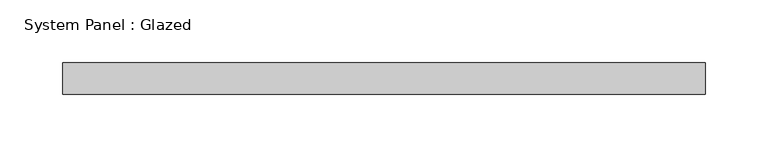
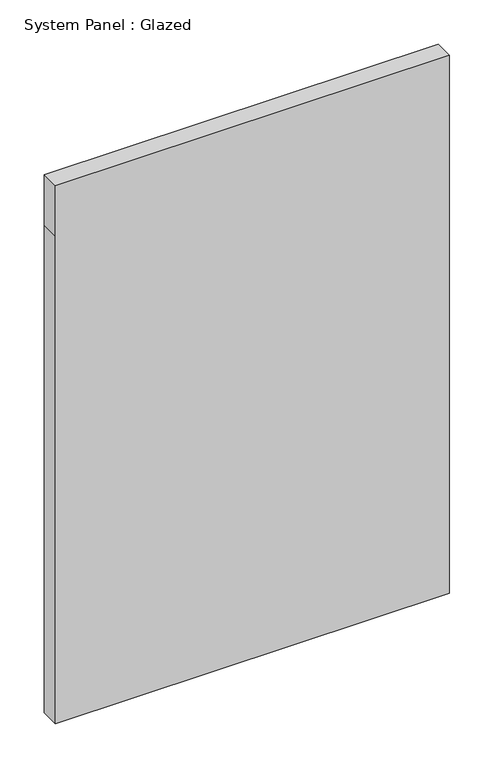
"""IFC4 building model written with IfcOpenShell, lengths in millimetres: plate geometry, System Panel : Glazed."""

from ifc_helpers import new_model, si_unit, frame, origin, place, context, project, spatial, polyline, outline, extrude, source, transform, mapped, element, save


def system_panel_glazed_bf274a97(model_context):
    return source(origin(), model_context, "Body", "SweptSolid", [
        extrude(outline(polyline([(0.0, -257.175), (0.0, 257.175), (672.7967564, 257.175), (742.6467564, 257.175), (742.6467564, -257.175), (672.7967564, -257.175), (0.0, -257.175)])), frame((0.0, 19.05, 0.0), z_axis=(0.0, 1.0, 0.0), x_axis=(0.0, 0.0, 1.0)), (0.0, 0.0, 1.0), 25.4),
    ])


if __name__ == "__main__":
    model = new_model("IFC4")
    model_context = context("Model", 3, world=origin())
    ifc_project = project(units=[si_unit("LENGTHUNIT", "METRE", prefix="MILLI")], contexts=[model_context])
    site = spatial("IfcSite", under=ifc_project)
    building = spatial("IfcBuilding", under=site)
    placement = place(None, origin())
    system_panel_glazed_shape = system_panel_glazed_bf274a97(model_context)
    element("IfcPlate", 1, ObjectType="System Panel : Glazed", at=placement, inside=building, context=model_context, shape_type="MappedRepresentation", body=[
        mapped(system_panel_glazed_shape, transform((0.0, 0.0, 0.0), x_axis=(1.0, 0.0, 0.0), y_axis=(0.0, 1.0, 0.0), z_axis=(0.0, 0.0, 1.0))),
    ])
    save(model, "model.ifc")

# Revit data of these elements
# Type "System Panel : Glazed"
#   Construction Type Id = "GSP4R"
#   Analytic Construction = "1/8 in Pilkington single glazing"
#   Visual Light Transmittance = 0.9
#   Solar Heat Gain Coefficient = 0.86
#   Heat Transfer Coefficient (U) = 1.18115 BTU/(h·ft²·°F)
#   Define Thermal Properties by = 1
# Element 1 (IfcPlate, "System Panel : Glazed")
#   Materials on its faces: "Glass"
# Materials
#   "Glass": class "Glass", colour RGB 0 128 192, transparency 0.75, Description = "Soda Lime Glass", Cost = 0
